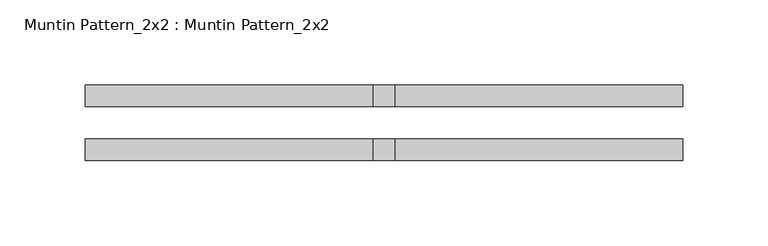
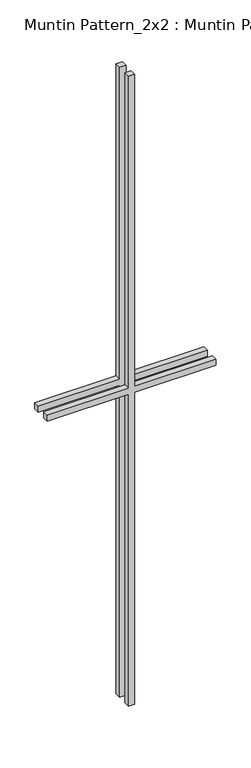
"""IFC4 building model written with IfcOpenShell, lengths in millimetres: proxy geometry, Muntin Pattern_2x2 : Muntin Pattern_2x2."""

from ifc_helpers import new_model, si_unit, frame, origin, place, context, project, spatial, polyline, outline, extrude, source, transform, mapped, element, save


def muntin_pattern_2x2_muntin_pattern_2x2_6cb77f41(model_context):
    return source(origin(), model_context, "Body", "SweptSolid", [
        extrude(outline(polyline([(698.5, -6.35), (698.5, -175.7591104), (685.8, -175.7591104), (685.8, -6.35), (0.0, -6.35), (0.0, 6.35), (685.8, 6.35), (685.8, 175.7591104), (698.5, 175.7591104), (698.5, 6.35), (1384.3, 6.35), (1384.3, -6.35), (698.5, -6.35)])), frame((0.0, -22.225, 0.0), z_axis=(0.0, 1.0, 0.0), x_axis=(0.0, 0.0, 1.0)), (0.0, 0.0, 1.0), 12.7),
        extrude(outline(polyline([(698.5, -6.35), (698.5, -175.7591104), (685.8, -175.7591104), (685.8, -6.35), (0.0, -6.35), (0.0, 6.35), (685.8, 6.35), (685.8, 175.7591104), (698.5, 175.7591104), (698.5, 6.35), (1384.3, 6.35), (1384.3, -6.35), (698.5, -6.35)])), frame((0.0, 9.525, 0.0), z_axis=(0.0, 1.0, 0.0), x_axis=(0.0, 0.0, 1.0)), (0.0, 0.0, 1.0), 12.7),
    ])


if __name__ == "__main__":
    model = new_model("IFC4")
    model_context = context("Model", 3, world=origin())
    ifc_project = project(units=[si_unit("LENGTHUNIT", "METRE", prefix="MILLI")], contexts=[model_context])
    site = spatial("IfcSite", under=ifc_project)
    building = spatial("IfcBuilding", under=site)
    placement = place(None, origin())
    muntin_pattern_2x2_muntin_pattern_2x2_shape = muntin_pattern_2x2_muntin_pattern_2x2_6cb77f41(model_context)
    element("IfcBuildingElementProxy", 1, Name="Muntin Pattern_2x2 : Muntin Pattern_2x2", ObjectType="Muntin Pattern_2x2 : Muntin Pattern_2x2", at=placement, inside=building, context=model_context, shape_type="MappedRepresentation", body=[
        mapped(muntin_pattern_2x2_muntin_pattern_2x2_shape, transform((0.0, 0.0, 0.0), x_axis=(1.0, 0.0, 0.0), y_axis=(0.0, 1.0, 0.0), z_axis=(0.0, 0.0, 1.0))),
    ])
    save(model, "model.ifc")

# Revit data of these elements
# Type "Muntin Pattern_2x2 : Muntin Pattern_2x2"
#   Width [instance default] = 4' - 0"
#   Thickness = 0' - 0 1/2"
#   Height [instance default] = 4' - 0"
#   Distance = 0' - 0 3/4"
#   Interior Material [instance default] = none
#   Exterior Material [instance default] = none
#   Default Elevation = 0
# Element 1 (IfcBuildingElementProxy, "Muntin Pattern_2x2 : Muntin Pattern_2x2")
#   Width = 1' - 1.8393"
#   Height = 4' - 6 1/2"
#   Interior Material = Wood - Stained
#   Exterior Material = Clad - White
#   Materials on its faces: "Clad - White", "Wood - Stained"
# Materials
#   "Clad - White": class "Wood", colour RGB 242 242 238, transparency 0, Cost = 0
#   "Wood - Stained": class "Wood", colour RGB 224 178 126, transparency 0, Cost = 0
